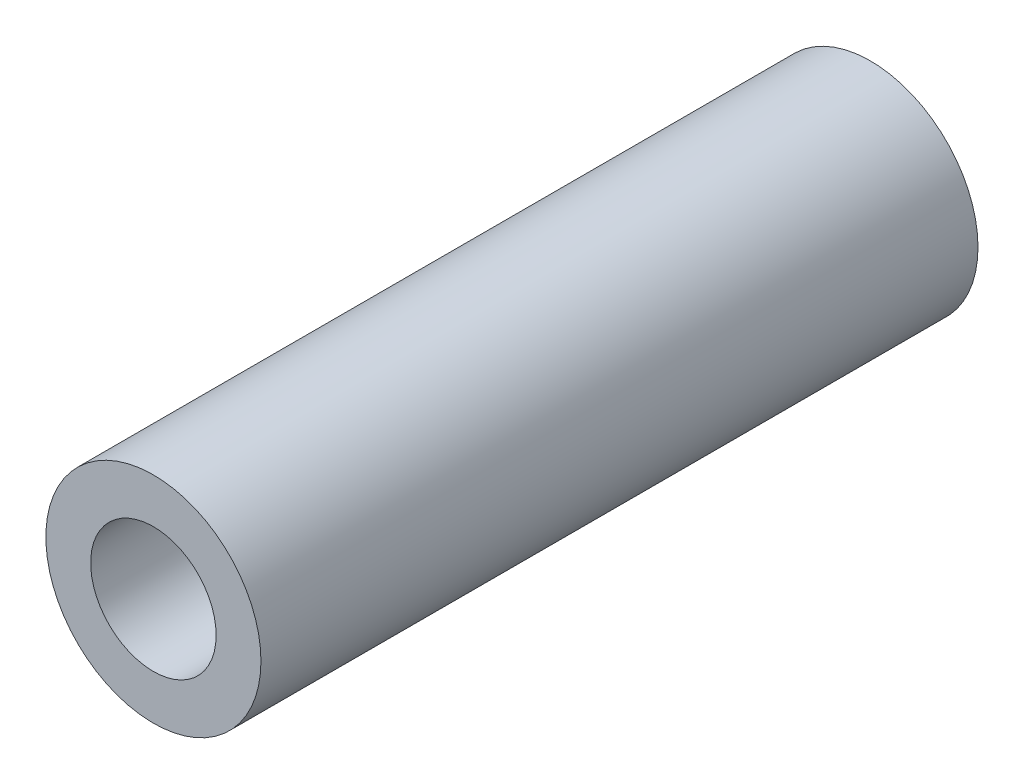
from build123d import *

# Parameters (mm, degrees)
BUSHING_PROFILE_6X_3_5_R   = 3
BUSHING_PROFILE_6X_3_5_R_2 = 1.75
BUSHING_BODY_L20_DEPTH     = 10


with BuildPart() as part:
    # Bushing Profile Ø6xØ3.5 → Bushing Body L20 (new, symmetric)
    with BuildSketch(Plane.XY):
        Circle(BUSHING_PROFILE_6X_3_5_R)
        Circle(BUSHING_PROFILE_6X_3_5_R_2, mode=Mode.SUBTRACT)
    extrude(amount=BUSHING_BODY_L20_DEPTH, both=True)


solid = part.part
